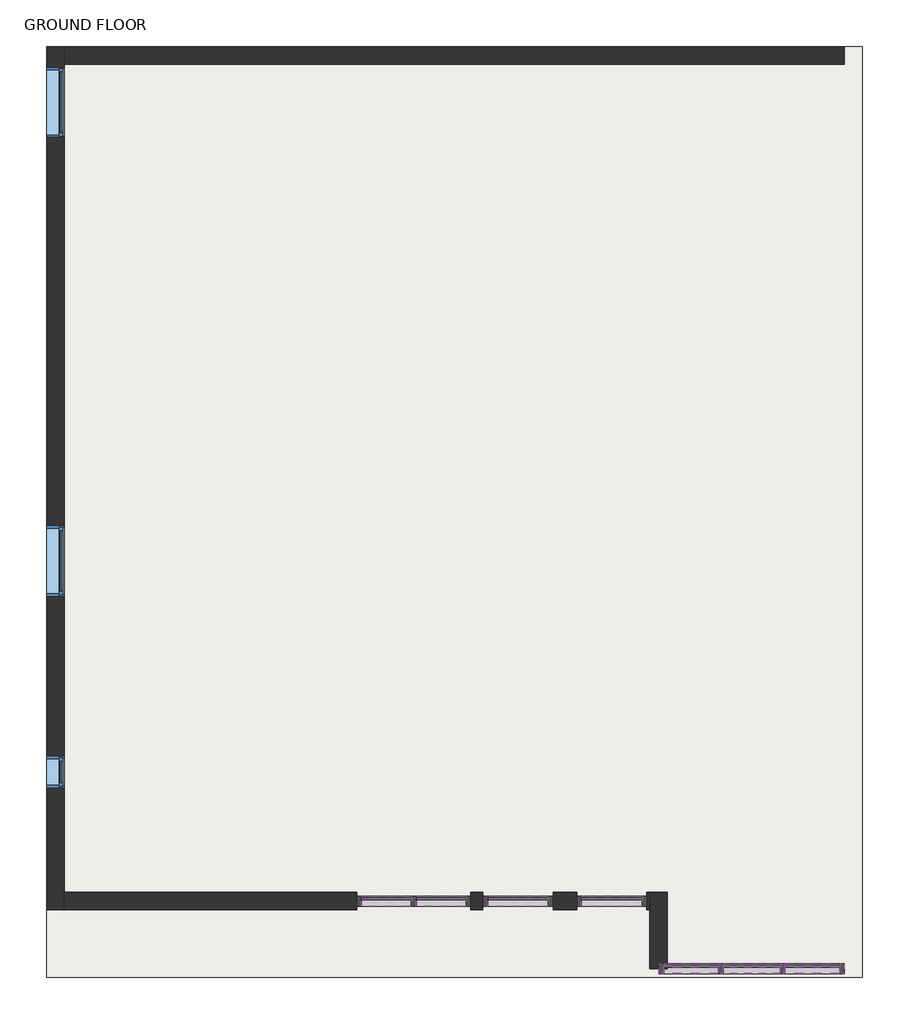
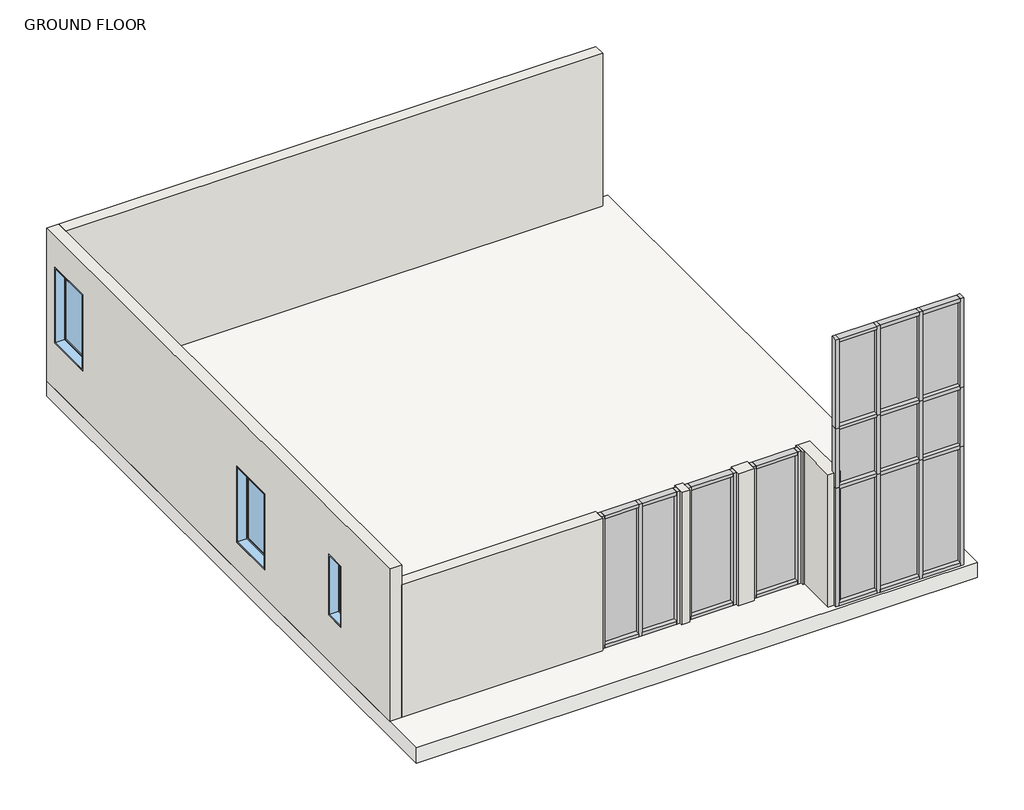
# One storey: 39 members, 13 plates, 7 walls, 3 windows, 1 slab.
"""IFC4 building model written with IfcOpenShell, lengths in millimetres."""

from ifc_helpers import new_model, si_unit, frame, origin, origin_with_axes, place, context, project, spatial, polyline, outline, extrude, faceted_brep, transform, mapped, element, save
from components import member_429f6687, member_3f28283e, member_1631f5ff, member_e606956e, member_f89ab80f, member_3301b6a7, member_46fef415, member_ec261fe8, member_e97ac6c9, member_8cc12096, member_fed28cdb, member_d1af338a, member_7df25b28, member_5215b92c, system_panel_glazed_923938e8, system_panel_glazed_b47d4196, system_panel_glazed_137e22aa, system_panel_glazed_161bf594, system_panel_glazed_5d718544, system_panel_glazed_0ba8262e, system_panel_glazed_6160ed8e, system_panel_glazed_744525f6, window_cea7027f, window_cd393ee1

model = new_model("IFC4")

# Units and contexts
model_context = context("Model", 3, world=origin())
ifc_project = project(units=[si_unit("LENGTHUNIT", "METRE", prefix="MILLI")], contexts=[model_context])

# Site, building, storey
site = spatial("IfcSite", under=ifc_project)
building = spatial("IfcBuilding", under=site)
storey = spatial("IfcBuildingStorey", under=building, Name="GROUND FLOOR", Elevation=0.0)

# Members
placement = place(None, origin())
member_shape = member_429f6687(model_context)
element("IfcMember", 1, ObjectType="Rectangular Mullion : 2.5\" x 5\" rectangular", at=placement, inside=storey, context=model_context, shape_type="MappedRepresentation", body=[
    mapped(member_shape, transform((-349.9207252, 1984.0953049, 2641.6), x_axis=(0.0, 0.0, 1.0), y_axis=(0.0, -1.0, 0.0), z_axis=(1.0, 0.0, 0.0))),
])
element("IfcMember", 2, ObjectType="Rectangular Mullion : 2.5\" x 5\" rectangular", at=placement, inside=storey, context=model_context, shape_type="MappedRepresentation", body=[
    mapped(member_shape, transform((869.2792748, 1984.0953049, 2641.6), x_axis=(0.0, 0.0, 1.0), y_axis=(0.0, -1.0, 0.0), z_axis=(1.0, 0.0, 0.0))),
])
element("IfcMember", 3, ObjectType="Rectangular Mullion : 2.5\" x 5\" rectangular", at=placement, inside=storey, context=model_context, shape_type="MappedRepresentation", body=[
    mapped(member_shape, transform((-1137.3207252, 1984.0953049, 0.0), x_axis=(0.0, 0.0, -1.0), y_axis=(0.0, -1.0, 0.0), z_axis=(-1.0, 0.0, 0.0))),
])
element("IfcMember", 4, ObjectType="Rectangular Mullion : 2.5\" x 5\" rectangular", at=placement, inside=storey, context=model_context, shape_type="MappedRepresentation", body=[
    mapped(member_shape, transform((81.8792748, 1984.0953049, 0.0), x_axis=(0.0, 0.0, -1.0), y_axis=(0.0, -1.0, 0.0), z_axis=(-1.0, 0.0, 0.0))),
])
member_2_shape = member_3f28283e(model_context)
element("IfcMember", 5, ObjectType="Rectangular Mullion : 2.5\" x 5\" rectangular", at=placement, inside=storey, context=model_context, shape_type="MappedRepresentation", body=[
    mapped(member_2_shape, transform((-1353.2207252, 1984.0953049, 0.0), x_axis=(1.0, 0.0, 0.0), y_axis=(0.0, -1.0, 0.0), z_axis=(0.0, 0.0, -1.0))),
])
element("IfcMember", 6, ObjectType="Rectangular Mullion : 2.5\" x 5\" rectangular", at=placement, inside=storey, context=model_context, shape_type="MappedRepresentation", body=[
    mapped(member_2_shape, transform((-286.4207252, 1984.0953049, 0.0), x_axis=(1.0, 0.0, 0.0), y_axis=(0.0, -1.0, 0.0), z_axis=(0.0, 0.0, -1.0))),
])
element("IfcMember", 7, ObjectType="Rectangular Mullion : 2.5\" x 5\" rectangular", at=placement, inside=storey, context=model_context, shape_type="MappedRepresentation", body=[
    mapped(member_2_shape, transform((932.7792748, 1984.0953049, 0.0), x_axis=(1.0, 0.0, 0.0), y_axis=(0.0, -1.0, 0.0), z_axis=(0.0, 0.0, -1.0))),
])
element("IfcMember", 8, ObjectType="Rectangular Mullion : 2.5\" x 5\" rectangular", at=placement, inside=storey, context=model_context, shape_type="MappedRepresentation", body=[
    mapped(member_2_shape, transform((-2839.1207252, 1984.0953049, 2641.6), x_axis=(-1.0, 0.0, 0.0), y_axis=(0.0, -1.0, 0.0), z_axis=(0.0, 0.0, 1.0))),
])
element("IfcMember", 9, ObjectType="Rectangular Mullion : 2.5\" x 5\" rectangular", at=placement, inside=storey, context=model_context, shape_type="MappedRepresentation", body=[
    mapped(member_2_shape, transform((-1200.8207252, 1984.0953049, 2641.6), x_axis=(-1.0, 0.0, 0.0), y_axis=(0.0, -1.0, 0.0), z_axis=(0.0, 0.0, 1.0))),
])
element("IfcMember", 10, ObjectType="Rectangular Mullion : 2.5\" x 5\" rectangular", at=placement, inside=storey, context=model_context, shape_type="MappedRepresentation", body=[
    mapped(member_2_shape, transform((18.3792748, 1984.0953049, 2641.6), x_axis=(-1.0, 0.0, 0.0), y_axis=(0.0, -1.0, 0.0), z_axis=(0.0, 0.0, 1.0))),
])
member_3_shape = member_1631f5ff(model_context)
element("IfcMember", 11, ObjectType="Rectangular Mullion : 2.5\" x 5\" rectangular", at=placement, inside=storey, context=model_context, shape_type="MappedRepresentation", body=[
    mapped(member_3_shape, transform((-2096.1707252, 1984.0953049, 0.0), x_axis=(1.0, 0.0, 0.0), y_axis=(0.0, -1.0, 0.0), z_axis=(0.0, 0.0, -1.0))),
])
member_4_shape = member_e606956e(model_context)
element("IfcMember", 12, ObjectType="Rectangular Mullion : 2.5\" x 5\" rectangular", at=placement, inside=storey, context=model_context, shape_type="MappedRepresentation", body=[
    mapped(member_4_shape, transform((1148.6792748, 1107.7953049, 0.0), x_axis=(0.0, 0.0, -1.0), y_axis=(0.0, -1.0, 0.0), z_axis=(-1.0, 0.0, 0.0))),
])
element("IfcMember", 13, ObjectType="Rectangular Mullion : 2.5\" x 5\" rectangular", at=placement, inside=storey, context=model_context, shape_type="MappedRepresentation", body=[
    mapped(member_4_shape, transform((2725.5376749, 1107.7953049, 0.0), x_axis=(0.0, 0.0, -1.0), y_axis=(0.0, -1.0, 0.0), z_axis=(-1.0, 0.0, 0.0))),
])
element("IfcMember", 14, ObjectType="Rectangular Mullion : 2.5\" x 5\" rectangular", at=placement, inside=storey, context=model_context, shape_type="MappedRepresentation", body=[
    mapped(member_4_shape, transform((3434.5918749, 1107.7953049, 5334.0), x_axis=(0.0, 0.0, 1.0), y_axis=(0.0, -1.0, 0.0), z_axis=(1.0, 0.0, 0.0))),
])
element("IfcMember", 15, ObjectType="Rectangular Mullion : 2.5\" x 5\" rectangular", at=placement, inside=storey, context=model_context, shape_type="MappedRepresentation", body=[
    mapped(member_4_shape, transform((1857.7334748, 1107.7953049, 5334.0), x_axis=(0.0, 0.0, 1.0), y_axis=(0.0, -1.0, 0.0), z_axis=(1.0, 0.0, 0.0))),
])
member_5_shape = member_f89ab80f(model_context)
element("IfcMember", 16, ObjectType="Rectangular Mullion : 2.5\" x 5\" rectangular", at=placement, inside=storey, context=model_context, shape_type="MappedRepresentation", body=[
    mapped(member_5_shape, transform((1921.2334748, 1107.7953049, 0.0), x_axis=(0.0, 0.0, -1.0), y_axis=(0.0, -1.0, 0.0), z_axis=(-1.0, 0.0, 0.0))),
])
element("IfcMember", 17, ObjectType="Rectangular Mullion : 2.5\" x 5\" rectangular", at=placement, inside=storey, context=model_context, shape_type="MappedRepresentation", body=[
    mapped(member_5_shape, transform((2662.0376749, 1107.7953049, 5334.0), x_axis=(0.0, 0.0, 1.0), y_axis=(0.0, -1.0, 0.0), z_axis=(1.0, 0.0, 0.0))),
])
member_6_shape = member_3301b6a7(model_context)
element("IfcMember", 18, ObjectType="Rectangular Mullion : 2.5\" x 5\" rectangular", at=placement, inside=storey, context=model_context, shape_type="MappedRepresentation", body=[
    mapped(member_6_shape, transform((1857.7334748, 1107.7953049, 3556.0), x_axis=(0.0, 0.0, 1.0), y_axis=(0.0, -1.0, 0.0), z_axis=(1.0, 0.0, 0.0))),
])
element("IfcMember", 19, ObjectType="Rectangular Mullion : 2.5\" x 5\" rectangular", at=placement, inside=storey, context=model_context, shape_type="MappedRepresentation", body=[
    mapped(member_6_shape, transform((3434.5918749, 1107.7953049, 3556.0), x_axis=(0.0, 0.0, 1.0), y_axis=(0.0, -1.0, 0.0), z_axis=(1.0, 0.0, 0.0))),
])
element("IfcMember", 20, ObjectType="Rectangular Mullion : 2.5\" x 5\" rectangular", at=placement, inside=storey, context=model_context, shape_type="MappedRepresentation", body=[
    mapped(member_6_shape, transform((1857.7334748, 1107.7953049, 2370.6666667), x_axis=(0.0, 0.0, 1.0), y_axis=(0.0, -1.0, 0.0), z_axis=(1.0, 0.0, 0.0))),
])
element("IfcMember", 21, ObjectType="Rectangular Mullion : 2.5\" x 5\" rectangular", at=placement, inside=storey, context=model_context, shape_type="MappedRepresentation", body=[
    mapped(member_6_shape, transform((3434.5918749, 1107.7953049, 2370.6666667), x_axis=(0.0, 0.0, 1.0), y_axis=(0.0, -1.0, 0.0), z_axis=(1.0, 0.0, 0.0))),
])
member_7_shape = member_46fef415(model_context)
element("IfcMember", 22, ObjectType="Rectangular Mullion : 2.5\" x 5\" rectangular", at=placement, inside=storey, context=model_context, shape_type="MappedRepresentation", body=[
    mapped(member_7_shape, transform((2662.0376749, 1107.7953049, 3556.0), x_axis=(0.0, 0.0, 1.0), y_axis=(0.0, -1.0, 0.0), z_axis=(1.0, 0.0, 0.0))),
])
element("IfcMember", 23, ObjectType="Rectangular Mullion : 2.5\" x 5\" rectangular", at=placement, inside=storey, context=model_context, shape_type="MappedRepresentation", body=[
    mapped(member_7_shape, transform((2662.0376749, 1107.7953049, 2370.6666667), x_axis=(0.0, 0.0, 1.0), y_axis=(0.0, -1.0, 0.0), z_axis=(1.0, 0.0, 0.0))),
])
member_8_shape = member_ec261fe8(model_context)
element("IfcMember", 24, ObjectType="Rectangular Mullion : 2.5\" x 5\" rectangular", at=placement, inside=storey, context=model_context, shape_type="MappedRepresentation", body=[
    mapped(member_8_shape, transform((1889.4834748, 1107.7953049, 3556.0), x_axis=(1.0, 0.0, 0.0), y_axis=(0.0, -1.0, 0.0), z_axis=(0.0, 0.0, -1.0))),
])
element("IfcMember", 25, ObjectType="Rectangular Mullion : 2.5\" x 5\" rectangular", at=placement, inside=storey, context=model_context, shape_type="MappedRepresentation", body=[
    mapped(member_8_shape, transform((2693.7876749, 1107.7953049, 3556.0), x_axis=(1.0, 0.0, 0.0), y_axis=(0.0, -1.0, 0.0), z_axis=(0.0, 0.0, -1.0))),
])
member_9_shape = member_e97ac6c9(model_context)
element("IfcMember", 26, ObjectType="Rectangular Mullion : 2.5\" x 5\" rectangular", at=placement, inside=storey, context=model_context, shape_type="MappedRepresentation", body=[
    mapped(member_9_shape, transform((1085.1792748, 1107.7953049, 5334.0), x_axis=(-1.0, 0.0, 0.0), y_axis=(0.0, -1.0, 0.0), z_axis=(0.0, 0.0, 1.0))),
])
element("IfcMember", 27, ObjectType="Rectangular Mullion : 2.5\" x 5\" rectangular", at=placement, inside=storey, context=model_context, shape_type="MappedRepresentation", body=[
    mapped(member_9_shape, transform((3498.0918749, 1107.7953049, 3556.0), x_axis=(1.0, 0.0, 0.0), y_axis=(0.0, -1.0, 0.0), z_axis=(0.0, 0.0, -1.0))),
])
member_10_shape = member_8cc12096(model_context)
element("IfcMember", 28, ObjectType="Rectangular Mullion : 2.5\" x 5\" rectangular", at=placement, inside=storey, context=model_context, shape_type="MappedRepresentation", body=[
    mapped(member_10_shape, transform((1889.4834748, 1107.7953049, 0.0), x_axis=(1.0, 0.0, 0.0), y_axis=(0.0, -1.0, 0.0), z_axis=(0.0, 0.0, -1.0))),
])
element("IfcMember", 29, ObjectType="Rectangular Mullion : 2.5\" x 5\" rectangular", at=placement, inside=storey, context=model_context, shape_type="MappedRepresentation", body=[
    mapped(member_10_shape, transform((2693.7876749, 1107.7953049, 0.0), x_axis=(1.0, 0.0, 0.0), y_axis=(0.0, -1.0, 0.0), z_axis=(0.0, 0.0, -1.0))),
])
member_11_shape = member_fed28cdb(model_context)
element("IfcMember", 30, ObjectType="Rectangular Mullion : 2.5\" x 5\" rectangular", at=placement, inside=storey, context=model_context, shape_type="MappedRepresentation", body=[
    mapped(member_11_shape, transform((1889.4834748, 1107.7953049, 2370.6666667), x_axis=(1.0, 0.0, 0.0), y_axis=(0.0, -1.0, 0.0), z_axis=(0.0, 0.0, -1.0))),
])
element("IfcMember", 31, ObjectType="Rectangular Mullion : 2.5\" x 5\" rectangular", at=placement, inside=storey, context=model_context, shape_type="MappedRepresentation", body=[
    mapped(member_11_shape, transform((2693.7876749, 1107.7953049, 2370.6666667), x_axis=(1.0, 0.0, 0.0), y_axis=(0.0, -1.0, 0.0), z_axis=(0.0, 0.0, -1.0))),
])
member_12_shape = member_d1af338a(model_context)
element("IfcMember", 32, ObjectType="Rectangular Mullion : 2.5\" x 5\" rectangular", at=placement, inside=storey, context=model_context, shape_type="MappedRepresentation", body=[
    mapped(member_12_shape, transform((3498.0918749, 1107.7953049, 0.0), x_axis=(1.0, 0.0, 0.0), y_axis=(0.0, -1.0, 0.0), z_axis=(0.0, 0.0, -1.0))),
])
member_13_shape = member_7df25b28(model_context)
element("IfcMember", 33, ObjectType="Rectangular Mullion : 2.5\" x 5\" rectangular", at=placement, inside=storey, context=model_context, shape_type="MappedRepresentation", body=[
    mapped(member_13_shape, transform((1085.1792748, 1107.7953049, 3556.0), x_axis=(-1.0, 0.0, 0.0), y_axis=(0.0, -1.0, 0.0), z_axis=(0.0, 0.0, 1.0))),
])
element("IfcMember", 34, ObjectType="Rectangular Mullion : 2.5\" x 5\" rectangular", at=placement, inside=storey, context=model_context, shape_type="MappedRepresentation", body=[
    mapped(member_13_shape, transform((3498.0918749, 1107.7953049, 2370.6666667), x_axis=(1.0, 0.0, 0.0), y_axis=(0.0, -1.0, 0.0), z_axis=(0.0, 0.0, -1.0))),
])
element("IfcMember", 35, ObjectType="Rectangular Mullion : 2.5\" x 5\" rectangular", at=placement, inside=storey, context=model_context, shape_type="MappedRepresentation", body=[
    mapped(member_12_shape, transform((1085.1792748, 1107.7953049, 2370.6666667), x_axis=(-1.0, 0.0, 0.0), y_axis=(0.0, -1.0, 0.0), z_axis=(0.0, 0.0, 1.0))),
])
member_14_shape = member_5215b92c(model_context)
element("IfcMember", 36, ObjectType="Rectangular Mullion : 2.5\" x 5\" rectangular", at=placement, inside=storey, context=model_context, shape_type="MappedRepresentation", body=[
    mapped(member_14_shape, transform((-1416.7207252, 1984.0953049, 2641.6), x_axis=(0.0, 0.0, 1.0), y_axis=(0.0, -1.0, 0.0), z_axis=(1.0, 0.0, 0.0))),
])
element("IfcMember", 37, ObjectType="Rectangular Mullion : 2.5\" x 5\" rectangular", at=placement, inside=storey, context=model_context, shape_type="MappedRepresentation", body=[
    mapped(member_14_shape, transform((-2127.9207252, 1984.0953049, 2641.6), x_axis=(0.0, 0.0, 1.0), y_axis=(0.0, -1.0, 0.0), z_axis=(1.0, 0.0, 0.0))),
])
element("IfcMember", 38, ObjectType="Rectangular Mullion : 2.5\" x 5\" rectangular", at=placement, inside=storey, context=model_context, shape_type="MappedRepresentation", body=[
    mapped(member_14_shape, transform((-2775.6207252, 1984.0953049, 0.0), x_axis=(0.0, 0.0, -1.0), y_axis=(0.0, -1.0, 0.0), z_axis=(-1.0, 0.0, 0.0))),
])
element("IfcMember", 39, ObjectType="Rectangular Mullion : 2.5\" x 5\" rectangular", at=placement, inside=storey, context=model_context, shape_type="MappedRepresentation", body=[
    mapped(member_14_shape, transform((-2064.4207252, 1984.0953049, 0.0), x_axis=(0.0, 0.0, -1.0), y_axis=(0.0, -1.0, 0.0), z_axis=(-1.0, 0.0, 0.0))),
])

# Plates
system_panel_glazed_shape = system_panel_glazed_923938e8(model_context)
element("IfcPlate", 40, ObjectType="System Panel : Glazed", at=placement, inside=storey, context=model_context, shape_type="MappedRepresentation", body=[
    mapped(system_panel_glazed_shape, transform((-743.6207252, 1984.0953049, 63.5), x_axis=(1.0, 0.0, 0.0), y_axis=(0.0, 1.0, 0.0), z_axis=(0.0, 0.0, 1.0))),
])
element("IfcPlate", 41, ObjectType="System Panel : Glazed", at=placement, inside=storey, context=model_context, shape_type="MappedRepresentation", body=[
    mapped(system_panel_glazed_shape, transform((475.5792748, 1984.0953049, 63.5), x_axis=(1.0, 0.0, 0.0), y_axis=(0.0, 1.0, 0.0), z_axis=(0.0, 0.0, 1.0))),
])
system_panel_glazed_2_shape = system_panel_glazed_b47d4196(model_context)
element("IfcPlate", 42, ObjectType="System Panel : Glazed", at=placement, inside=storey, context=model_context, shape_type="MappedRepresentation", body=[
    mapped(system_panel_glazed_2_shape, transform((1503.2063748, 1107.7953049, 3587.75), x_axis=(1.0, 0.0, 0.0), y_axis=(0.0, 1.0, 0.0), z_axis=(0.0, 0.0, 1.0))),
])
element("IfcPlate", 43, ObjectType="System Panel : Glazed", at=placement, inside=storey, context=model_context, shape_type="MappedRepresentation", body=[
    mapped(system_panel_glazed_2_shape, transform((3080.0647749, 1107.7953049, 3587.75), x_axis=(1.0, 0.0, 0.0), y_axis=(0.0, 1.0, 0.0), z_axis=(0.0, 0.0, 1.0))),
])
system_panel_glazed_3_shape = system_panel_glazed_137e22aa(model_context)
element("IfcPlate", 44, ObjectType="System Panel : Glazed", at=placement, inside=storey, context=model_context, shape_type="MappedRepresentation", body=[
    mapped(system_panel_glazed_3_shape, transform((2291.6355748, 1107.7953049, 3587.75), x_axis=(1.0, 0.0, 0.0), y_axis=(0.0, 1.0, 0.0), z_axis=(0.0, 0.0, 1.0))),
])
system_panel_glazed_4_shape = system_panel_glazed_161bf594(model_context)
element("IfcPlate", 45, ObjectType="System Panel : Glazed", at=placement, inside=storey, context=model_context, shape_type="MappedRepresentation", body=[
    mapped(system_panel_glazed_4_shape, transform((1503.2063748, 1107.7953049, 63.5), x_axis=(1.0, 0.0, 0.0), y_axis=(0.0, 1.0, 0.0), z_axis=(0.0, 0.0, 1.0))),
])
element("IfcPlate", 46, ObjectType="System Panel : Glazed", at=placement, inside=storey, context=model_context, shape_type="MappedRepresentation", body=[
    mapped(system_panel_glazed_4_shape, transform((3080.0647749, 1107.7953049, 63.5), x_axis=(1.0, 0.0, 0.0), y_axis=(0.0, 1.0, 0.0), z_axis=(0.0, 0.0, 1.0))),
])
system_panel_glazed_5_shape = system_panel_glazed_5d718544(model_context)
element("IfcPlate", 47, ObjectType="System Panel : Glazed", at=placement, inside=storey, context=model_context, shape_type="MappedRepresentation", body=[
    mapped(system_panel_glazed_5_shape, transform((2291.6355748, 1107.7953049, 63.5), x_axis=(1.0, 0.0, 0.0), y_axis=(0.0, 1.0, 0.0), z_axis=(0.0, 0.0, 1.0))),
])
system_panel_glazed_6_shape = system_panel_glazed_0ba8262e(model_context)
element("IfcPlate", 48, ObjectType="System Panel : Glazed", at=placement, inside=storey, context=model_context, shape_type="MappedRepresentation", body=[
    mapped(system_panel_glazed_6_shape, transform((1503.2063748, 1107.7953049, 2402.4166667), x_axis=(1.0, 0.0, 0.0), y_axis=(0.0, 1.0, 0.0), z_axis=(0.0, 0.0, 1.0))),
])
element("IfcPlate", 49, ObjectType="System Panel : Glazed", at=placement, inside=storey, context=model_context, shape_type="MappedRepresentation", body=[
    mapped(system_panel_glazed_6_shape, transform((3080.0647749, 1107.7953049, 2402.4166667), x_axis=(1.0, 0.0, 0.0), y_axis=(0.0, 1.0, 0.0), z_axis=(0.0, 0.0, 1.0))),
])
system_panel_glazed_7_shape = system_panel_glazed_6160ed8e(model_context)
element("IfcPlate", 50, ObjectType="System Panel : Glazed", at=placement, inside=storey, context=model_context, shape_type="MappedRepresentation", body=[
    mapped(system_panel_glazed_7_shape, transform((2291.6355748, 1107.7953049, 2402.4166667), x_axis=(1.0, 0.0, 0.0), y_axis=(0.0, 1.0, 0.0), z_axis=(0.0, 0.0, 1.0))),
])
system_panel_glazed_8_shape = system_panel_glazed_744525f6(model_context)
element("IfcPlate", 51, ObjectType="System Panel : Glazed", at=placement, inside=storey, context=model_context, shape_type="MappedRepresentation", body=[
    mapped(system_panel_glazed_8_shape, transform((-2451.7707252, 1984.0953049, 63.5), x_axis=(1.0, 0.0, 0.0), y_axis=(0.0, 1.0, 0.0), z_axis=(0.0, 0.0, 1.0))),
])
element("IfcPlate", 52, ObjectType="System Panel : Glazed", at=placement, inside=storey, context=model_context, shape_type="MappedRepresentation", body=[
    mapped(system_panel_glazed_8_shape, transform((-1740.5707252, 1984.0953049, 63.5), x_axis=(1.0, 0.0, 0.0), y_axis=(0.0, 1.0, 0.0), z_axis=(0.0, 0.0, 1.0))),
])

# Slab
element("IfcSlab", 53, ObjectType="Generic - 12\"", at=placement, inside=storey, context=model_context, shape_type="SweptSolid", body=[
    extrude(outline(polyline([(3726.6918749, 13083.8953049), (3726.6918749, 993.4953049), (-6865.1081251, 993.4953049), (-6865.1081251, 13083.8953049), (3726.6918749, 13083.8953049)])), frame((0.0, 0.0, -304.8), z_axis=(0.0, 0.0, 1.0), x_axis=(1.0, 0.0, 0.0)), (0.0, 0.0, 1.0), 304.8),
])

# Walls
element("IfcWall", 54, ObjectType="9\"", at=placement, inside=storey, context=model_context, shape_type="Brep", body=[
    faceted_brep([(-6636.5081251, 1869.7953049, 0.0), (-6636.5081251, 2098.3953049, 0.0), (-6636.5081251, 12855.2953049, 0.0), (-6636.5081251, 13083.8953049, 0.0), (-6636.5081251, 13083.8953049, 3048.0), (-6636.5081251, 12855.2953049, 3048.0), (-6636.5081251, 1869.7953049, 3048.0), (-6636.5081251, 1869.7953049, 2641.6), (-6636.5081251, 5946.4953049, 2074.3622584), (-6636.5081251, 6860.8953049, 2074.3622584), (-6636.5081251, 6860.8953049, 550.3622584), (-6636.5081251, 5946.4953049, 550.3622584), (-6636.5081251, 11902.7953049, 2438.4), (-6636.5081251, 12817.1953049, 2438.4), (-6636.5081251, 12817.1953049, 914.4), (-6636.5081251, 11902.7953049, 914.4), (-6636.5081251, 3457.2953049, 2133.6), (-6636.5081251, 3863.6953049, 2133.6), (-6636.5081251, 3863.6953049, 914.4), (-6636.5081251, 3457.2953049, 914.4), (-6865.1081251, 1869.7953049, 0.0), (-6865.1081251, 1869.7953049, 3048.0), (-6865.1081251, 13083.8953049, 3048.0), (-6865.1081251, 13083.8953049, 0.0), (-6865.1081251, 5946.4953049, 2074.3622584), (-6865.1081251, 5946.4953049, 550.3622584), (-6865.1081251, 6860.8953049, 550.3622584), (-6865.1081251, 6860.8953049, 2074.3622584), (-6865.1081251, 11902.7953049, 2438.4), (-6865.1081251, 11902.7953049, 914.4), (-6865.1081251, 12817.1953049, 914.4), (-6865.1081251, 12817.1953049, 2438.4), (-6865.1081251, 3457.2953049, 2133.6), (-6865.1081251, 3457.2953049, 914.4), (-6865.1081251, 3863.6953049, 914.4), (-6865.1081251, 3863.6953049, 2133.6)], [[[0, 1, 2, 3, 4, 5, 6, 7], [8, 9, 10, 11], [12, 13, 14, 15], [16, 17, 18, 19]], [[20, 21, 22, 23], [24, 25, 26, 27], [28, 29, 30, 31], [32, 33, 34, 35]], [[3, 2, 1, 0, 20, 23]], [[6, 5, 4, 22, 21]], [[4, 3, 23, 22]], [[0, 7, 6, 21, 20]], [[25, 24, 8, 11]], [[26, 25, 11, 10]], [[27, 26, 10, 9]], [[24, 27, 9, 8]], [[29, 28, 12, 15]], [[30, 29, 15, 14]], [[31, 30, 14, 13]], [[28, 31, 13, 12]], [[33, 32, 16, 19]], [[34, 33, 19, 18]], [[35, 34, 18, 17]], [[32, 35, 17, 16]]]),
])
element("IfcWall", 55, ObjectType="9\"", at=placement, inside=storey, context=model_context, shape_type="SweptSolid", body=[
    extrude(outline(polyline([(3498.0918749, 12855.2953049), (-6636.5081251, 12855.2953049), (-6636.5081251, 13083.8953049), (3498.0918749, 13083.8953049), (3498.0918749, 12855.2953049)])), origin_with_axes(), (0.0, 0.0, 1.0), 3048.0),
])
element("IfcWall", 56, ObjectType="9\"", at=placement, inside=storey, context=model_context, shape_type="Brep", body=[
    faceted_brep([(1199.4792748, 1107.7953049, 0.0), (1199.4792748, 2098.3953049, 0.0), (1199.4792748, 2098.3953049, 2641.6), (1199.4792748, 1107.7953049, 2641.6), (970.8792748, 1107.7953049, 0.0), (970.8792748, 1107.7953049, 2641.6), (970.8792748, 1869.7953049, 2641.6), (970.8792748, 2098.3953049, 2641.6), (970.8792748, 2098.3953049, 0.0), (970.8792748, 1869.7953049, 0.0)], [[[0, 1, 2, 3]], [[4, 5, 6, 7, 8, 9]], [[1, 0, 4, 9, 8]], [[3, 2, 7, 6, 5]], [[0, 3, 5, 4]], [[2, 1, 8, 7]]]),
])
element("IfcWall", 57, ObjectType="9\"", at=placement, inside=storey, context=model_context, shape_type="SweptSolid", body=[
    extrude(outline(polyline([(932.7792748, 2098.3953049), (970.8792748, 2098.3953049), (970.8792748, 1869.7953049), (932.7792748, 1869.7953049), (932.7792748, 2098.3953049)])), origin_with_axes(), (0.0, 0.0, 1.0), 2641.6),
])
element("IfcWall", 58, ObjectType="9\"", at=placement, inside=storey, context=model_context, shape_type="SweptSolid", body=[
    extrude(outline(polyline([(-286.4207252, 2098.3953049), (18.3792748, 2098.3953049), (18.3792748, 1869.7953049), (-286.4207252, 1869.7953049), (-286.4207252, 2098.3953049)])), origin_with_axes(), (0.0, 0.0, 1.0), 2641.6),
])
element("IfcWall", 59, ObjectType="9\"", at=placement, inside=storey, context=model_context, shape_type="SweptSolid", body=[
    extrude(outline(polyline([(-1353.2207252, 2098.3953049), (-1200.8207252, 2098.3953049), (-1200.8207252, 1869.7953049), (-1353.2207252, 1869.7953049), (-1353.2207252, 2098.3953049)])), origin_with_axes(), (0.0, 0.0, 1.0), 2641.6),
])
element("IfcWall", 60, ObjectType="9\"", at=placement, inside=storey, context=model_context, shape_type="SweptSolid", body=[
    extrude(outline(polyline([(-6636.5081251, 2098.3953049), (-2839.1207252, 2098.3953049), (-2839.1207252, 1869.7953049), (-6636.5081251, 1869.7953049), (-6636.5081251, 2098.3953049)])), origin_with_axes(), (0.0, 0.0, 1.0), 2641.6),
])

# Windows
window_shape = window_cea7027f(model_context)
element("IfcWindow", 61, ObjectType="Fixed : 16\" x 48\"", at=placement, inside=storey, context=model_context, shape_type="MappedRepresentation", body=[
    mapped(window_shape, transform((-6750.8081251, 3622.3953049, 0.0), x_axis=(0.0, -1.0, 0.0), y_axis=(1.0, 0.0, 0.0), z_axis=(0.0, 0.0, 1.0))),
])
window_2_shape = window_cd393ee1(model_context)
element("IfcWindow", 62, ObjectType="Fixed : 36\" x 48\"", at=placement, inside=storey, context=model_context, shape_type="MappedRepresentation", body=[
    mapped(window_2_shape, transform((-6750.8081251, 6365.5953049, -364.0377416), x_axis=(0.0, -1.0, 0.0), y_axis=(1.0, 0.0, 0.0), z_axis=(0.0, 0.0, 1.0))),
])
element("IfcWindow", 63, ObjectType="Fixed : 36\" x 48\"", at=placement, inside=storey, context=model_context, shape_type="MappedRepresentation", body=[
    mapped(window_2_shape, transform((-6750.8081251, 12321.8953049, 0.0), x_axis=(0.0, -1.0, 0.0), y_axis=(1.0, 0.0, 0.0), z_axis=(0.0, 0.0, 1.0))),
])

save(model, "model.ifc")

# Revit data of these elements
# Type "Rectangular Mullion : 2.5\" x 5\" rectangular"
#   built-in parameter 1007304 = 0.416667 (stored number, unit not read)
#   built-in parameter 1007301 = 0.104167 (stored number, unit not read)
#   built-in parameter 1007300 = 0.104167 (stored number, unit not read)
# Type "System Panel : Glazed"
#   Construction Type Id = "GSP4R"
#   Analytic Construction = "1/8 in Pilkington single glazing"
#   Visual Light Transmittance = 0.9
#   Solar Heat Gain Coefficient = 0.86
#   Heat Transfer Coefficient (U) = 1.18115 BTU/(h·ft²·°F)
#   Define Thermal Properties by = 1
# Type "Generic - 12\""
#   Assembly Code = "B1010"
#   Function = 0
#   Layers, outside or top first: 1' - 0" no material (function 1)
# Type "9\""
#   Assembly Code = "B2010"
#   Layers, outside or top first: 0' - 9" "1 wall" (function 1)
# Type "Fixed : 16\" x 48\""
#   Type Mark = "5"
#   Construction Type Id = "GSP4R"
#   Assembly Code = "B2020100"
#   Analytic Construction = "1/8 in Pilkington single glazing"
#   Visual Light Transmittance = 0.9
#   Solar Heat Gain Coefficient = 0.78
#   Heat Transfer Coefficient (U) = 0.6496 BTU/(h·ft²·°F)
#   Height = 4' - 0"
#   Default Sill Height = 3' - 0"
#   Width = 1' - 4"
#   Window Inset = 0' - 0 3/4"
#   Define Thermal Properties by = 1
#   Define Thermal Properties by = 1
#   Glass Pane Material = Glass
#   Sash Material = Sash
#   Wall Closure = (empty or 0)
# Type "Fixed : 36\" x 48\""
#   Type Mark = "1"
#   Construction Type Id = "GSP4R"
#   Assembly Code = "B2020100"
#   Analytic Construction = "1/8 in Pilkington single glazing"
#   Visual Light Transmittance = 0.9
#   Solar Heat Gain Coefficient = 0.78
#   Heat Transfer Coefficient (U) = 0.6496 BTU/(h·ft²·°F)
#   Height = 5' - 0"
#   Default Sill Height = 3' - 0"
#   Width = 3' - 0"
#   Window Inset = 0' - 0 3/4"
#   Define Thermal Properties by = 1
#   Define Thermal Properties by = 1
#   Glass Pane Material = Glass
#   Sash Material = Sash
#   Wall Closure = (empty or 0)
# Elements 1, 2, 3, 4, 5, 6, 7, 8, 9, 10, 11, 12, 13, 14, 15, 16, 17, 18, 19, 20, 21, 22, 23, 24, 25, 26, 27, 28, 29, 30, 31, 32, 33, 34, 35, 36, 37, 38, 39 (IfcMember, "Rectangular Mullion : 2.5\" x 5\" rectangular")
#   Phase Created = New Construction
#   Materials on its faces: "Aluminum"
# Elements 40, 41, 42, 43, 44, 45, 46, 47, 48, 49, 50, 51, 52 (IfcPlate, "System Panel : Glazed")
#   Phase Created = New Construction
#   Materials on its faces: "Glass"
# Element 53 (IfcSlab, "Generic - 12\"")
#   Height Offset From Level = 0' - 0"
#   Phase Created = New Construction
#   Materials on its faces: "Default Floor", "1 white", "Acoustic Ceiling Tile 24 x 24"
# Elements 54, 55 (IfcWall, "9\"")
#   Top Offset = 0' - 0"
#   Base Offset = 0' - 0"
#   Unconnected Height = 10' - 0"
#   wall height = 10' - 0"
#   Phase Created = New Construction
#   Base Constraint = GROUND FLOOR
#   Materials on its faces: "1 wall"
# Elements 56, 57, 58, 59, 60 (IfcWall, "9\"")
#   Top Offset = 0' - 0"
#   Base Offset = 0' - 0"
#   Unconnected Height = 8' - 8"
#   wall height = 8' - 8"
#   Phase Created = New Construction
#   Base Constraint = GROUND FLOOR
#   Materials on its faces: "1 wall"
# Element 61 (IfcWindow, "Fixed : 16\" x 48\"")
#   Mark = "6"
#   Phase Created = New Construction
#   Materials on its faces: "Sash", "Glass"
# Element 62 (IfcWindow, "Fixed : 36\" x 48\"")
#   Mark = "4"
#   Phase Created = New Construction
#   Materials on its faces: "Sash", "Glass"
# Element 63 (IfcWindow, "Fixed : 36\" x 48\"")
#   Mark = "5"
#   Phase Created = New Construction
#   Materials on its faces: "Sash", "Glass"
# Materials
#   "1 wall": class "Generic", colour RGB 172 157 136, transparency 0, Cost = 0
#   "Glass": class "Glass", colour RGB 0 128 192, transparency 0.75, Description = "Soda Lime Glass", Cost = 0
#   "Sash": class "Wood", colour RGB 224 178 126, transparency 0, Cost = 0
#   "Aluminum": class "Metal", colour RGB 247 247 247, transparency 0, Description = "Aluminum 6061", Cost = 0
#   "Default Floor": colour RGB 128 128 128, transparency 0, Cost = 0
#   "1 white": class "Generic", colour RGB 244 245 241, transparency 0, Cost = 0
#   "Acoustic Ceiling Tile 24 x 24": class "Generic", colour RGB 232 232 232, transparency 0, Description = "Acoustic Ceiling Tile 24 x 24", Cost = 0
